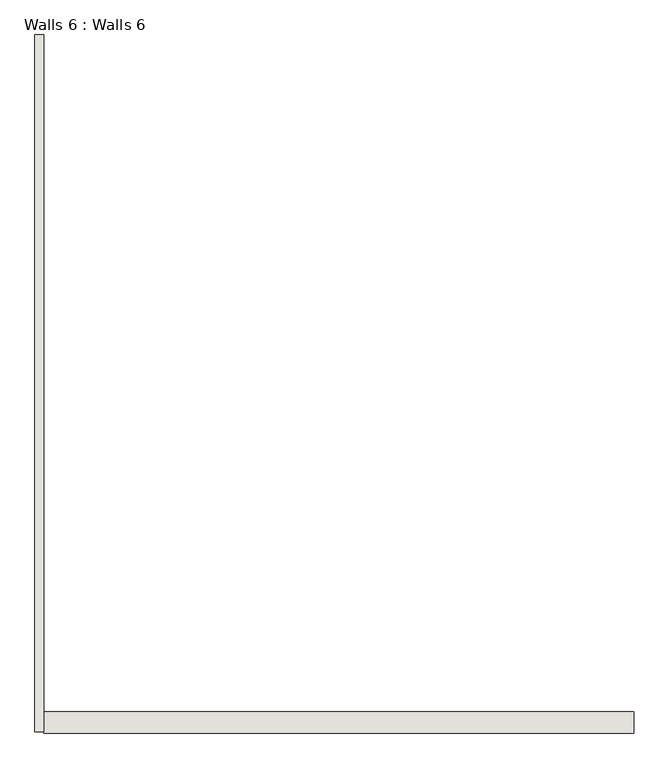
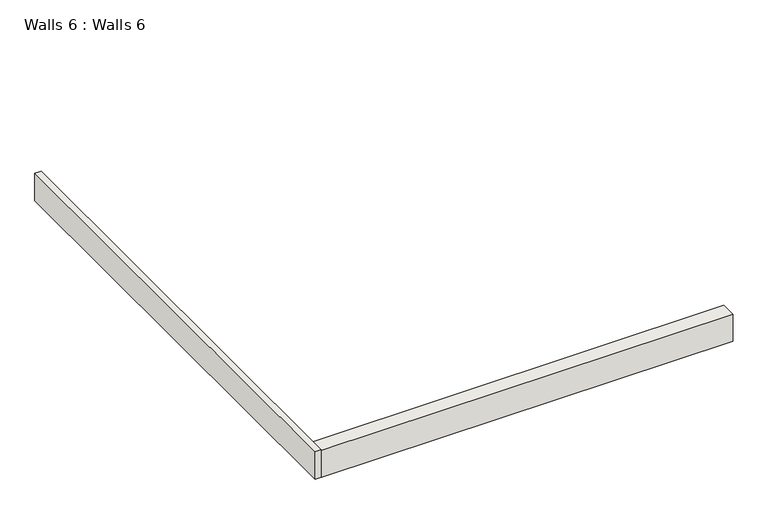
"""IFC4 building model written with IfcOpenShell, lengths in millimetres: wall geometry, Walls 6 : Walls 6."""

from ifc_helpers import new_model, si_unit, frame, origin, place, context, project, spatial, polyline, outline, extrude, source, transform, mapped, element, save


def walls_6_walls_6_29cd6f88(model_context):
    return source(origin(), model_context, "Body", "SweptSolid", [
        extrude(outline(polyline([(-9035.1322393, -4294.0325754), (-9035.1322393, 9625.1674246), (-8860.5727738, 9625.1674246), (-8860.5727738, -4294.0325754), (-9035.1322393, -4294.0325754)])), frame((0.0, 0.0, 3127.1876432), z_axis=(0.0, 0.0, 1.0), x_axis=(1.0, 0.0, 0.0)), (0.0, 0.0, 1.0), 835.2123568),
        extrude(outline(polyline([(2919.675018, -4315.9183249), (-8860.5727738, -4315.9183249), (-8860.5727738, -3887.6325754), (2919.675018, -3887.6325754), (2919.675018, -4315.9183249)])), frame((0.0, 0.0, 3135.1819058), z_axis=(0.0, 0.0, 1.0), x_axis=(1.0, 0.0, 0.0)), (0.0, 0.0, 1.0), 827.2180942),
    ])


if __name__ == "__main__":
    model = new_model("IFC4")
    model_context = context("Model", 3, world=origin())
    ifc_project = project(units=[si_unit("LENGTHUNIT", "METRE", prefix="MILLI")], contexts=[model_context])
    site = spatial("IfcSite", under=ifc_project)
    building = spatial("IfcBuilding", under=site)
    placement = place(None, origin())
    walls_6_walls_6_shape = walls_6_walls_6_29cd6f88(model_context)
    element("IfcWall", 1, ObjectType="Walls 6 : Walls 6", at=placement, inside=building, context=model_context, shape_type="MappedRepresentation", body=[
        mapped(walls_6_walls_6_shape, transform((0.0, 0.0, 0.0), x_axis=(1.0, 0.0, 0.0), y_axis=(0.0, 1.0, 0.0), z_axis=(0.0, 0.0, 1.0))),
    ])
    save(model, "model.ifc")

# Revit data of these elements
# Element 1 (IfcWall, "Walls 6 : Walls 6")
#   Materials on its faces: "Default Wall"
# Materials
#   "Default Wall": colour RGB 128 128 128, transparency 0
